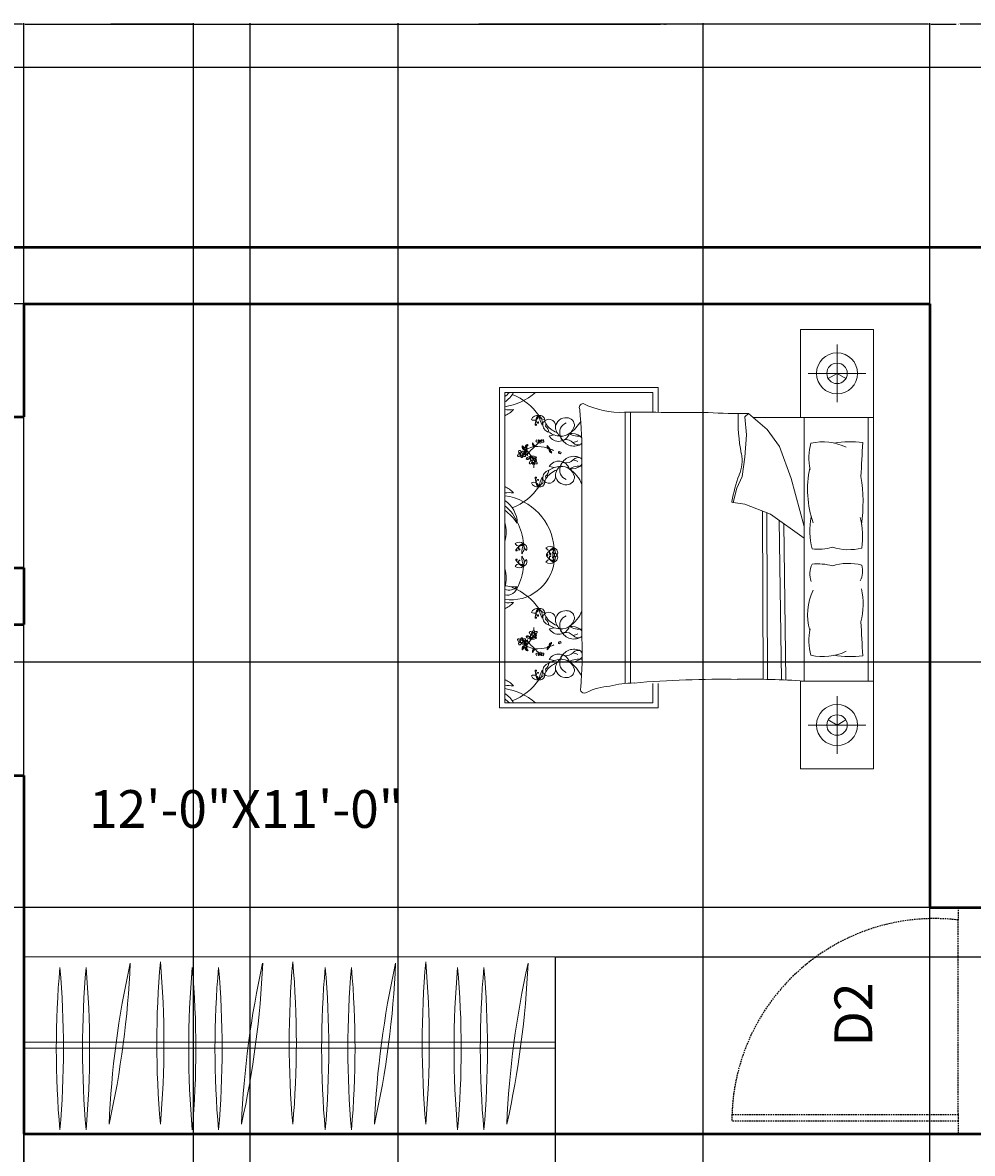
# Model space of a CAD drawing. Units: inches. Extents: x 3 to 576, y -689 to 51.
# Tile 17 of 21: x 111 to 262, y -128 to 51. Entities that reach past the tile are written whole.
import ezdxf

# ---------------------------------------------------------------- set-up
doc = ezdxf.new("R2010")
doc.units = ezdxf.units.IN
doc.header["$MEASUREMENT"] = 0
doc.linetypes.add('DASHED2', pattern=[0.375, 0.25, -0.125])
for name, color, linetype, lineweight in [('A-ANNO-DIMS', 2, 'Continuous', 18), ('A-ANNO-TEXT', 3, 'Continuous', 18), ('A-AREA-IDEN', 7, 'Continuous', 18), ('A-DOOR', 4, 'DASHED2', 25), ('A-FURN', 8, 'Continuous', 18), ('A-WALL', 7, 'Continuous', 50)]:
    doc.layers.add(name, color=color, linetype=linetype, lineweight=lineweight)
doc.styles.get("Standard").update_dxf_attribs({"font": 'arial.ttf'})
doc.dimstyles.get("Standard").update_dxf_attribs({"dimtxt": 0.18, "dimasz": 0.18, "dimexe": 0.18, "dimexo": 0.0625, "dimgap": 0.09, "dimtad": 0, "dimtih": 1, "dimtoh": 1, "dimdec": 0, "dimzin": 0, "dimdsep": 46, "dimlunit": 3, "dimtxsty": 'Standard', "dimcen": 0.09, "dimadec": 0, "dimazin": 0, "dimtfac": 1, "dimtdec": 0, "dimtofl": 0, "dimtmove": 0, "dimatfit": 3, "dimfxl": 1, "dimtolj": 1, "dimtzin": 0, "dimarcsym": 0})

# ---------------------------------------------------------------- blocks, each defined once
blk = doc.blocks.new('*D1')
at = {"layer": 'A-ANNO-DIMS', "color": 0, "lineweight": -2, "transparency": 16777216}
for p, q in [((38.29, 15.75), (38.29, 44.49)), ((38.47, 44.31), (276.45, 44.31)), ((540.11, 44.31), (302.14, 44.31)), ((540.29, 15.75), (540.29, 44.49))]:
    blk.add_line(p, q, dxfattribs=at)
at = {"layer": 'A-ANNO-DIMS', "color": 0, "transparency": 16777216}
for points in [[(38.47, 44.34), (38.47, 44.28), (38.29, 44.31)], [(540.11, 44.34), (540.11, 44.28), (540.29, 44.31)]]:
    blk.add_solid(points, dxfattribs=at)
at = {"layer": 'Defpoints', "color": 0, "transparency": 16777216}
for p in [(540.29, 44.31), (38.29, 15.69), (540.29, 15.69)]:
    blk.add_point(p, dxfattribs=at)
at = {"layer": 'A-ANNO-DIMS', "color": 0, "transparency": 16777216, "insert": (289.29, 44.31), "char_height": 6, "attachment_point": 5}
blk.add_mtext('\\A1;41\'-10"', dxfattribs=at)
blk = doc.blocks.new('BED-DOUBLE')
for p, q in [((59.45, 69.91), (59.45, 0)), ((53.63, 58.35), (53.63, 67.49)), ((49.06, 62.92), (58.2, 62.92)), ((0, 60.68), (25.18, 60.68)), ((0, 9.72), (0, 60.68)), ((0.81, 59.87), (0.81, 10.53)), ((24.37, 59.87), (0.81, 59.87)), ((24.37, 56.73), (24.37, 59.87)), ((25.18, 60.68), (25.18, 56.73)), ((19.95, 13.6), (19.95, 56.73)), ((20.82, 13.66), (20.82, 56.73)), ((38.97, 55.99), (39.54, 56.55)), ((39.25, 53.16), (38.97, 55.99)), ((39.54, 56.55), (42.51, 54.01)), ((59.45, 55.93), (40.27, 55.93)), ((48.41, 55.93), (48.41, 13.98)), ((58.56, 13.98), (58.56, 55.93)), ((42.51, 54.01), (44.49, 51.31)), ((7.9, 52.98), (8.69, 53.14)), ((38.97, 49.62), (39.25, 53.16)), ((44.49, 51.31), (46.33, 46.22)), ((13.08, 20.76), (13.08, 49.15)), ((38.55, 46.5), (38.97, 49.62)), ((7.9, 48.1), (8.69, 47.94)), ((37.7, 44.66), (38.55, 46.5)), ((46.33, 46.22), (48.41, 38.59)), ((37.13, 42.39), (37.7, 44.66)), ((38.97, 42.11), (37.13, 42.39)), ((43.07, 40.55), (38.97, 42.11)), ((41.87, 14.23), (41.76, 41.05)), ((42.58, 14.23), (42.48, 40.78)), ((48.41, 36.72), (43.07, 40.55)), ((44.78, 14.2), (44.43, 39.58)), ((45.5, 14.17), (45.15, 39.06)), ((7.9, 22.3), (8.69, 22.46)), ((7.9, 17.41), (8.69, 17.26)), ((24.37, 10.53), (24.37, 13.61)), ((25.18, 13.59), (25.18, 9.72)), ((53.63, 11.56), (53.63, 2.42)), ((25.18, 9.72), (0, 9.72)), ((0.81, 10.53), (24.37, 10.53)), ((49.06, 6.99), (58.2, 6.99))]:
    blk.add_line(p, q)
for points in [[(47.8, 55.93), (47.8, 69.91), (59.45, 69.91)], [(53.63, 62.92), (52.22, 62.1)], [(53.63, 62.92), (55.04, 62.1)], [(59.45, 13.98), (47.8, 13.98), (47.8, 0), (59.45, 0)], [(53.63, 6.99), (52.22, 7.81)], [(53.63, 6.99), (55.04, 7.81)]]:
    blk.add_lwpolyline(points)
for points in [[(33.13, 56.7, 0.001242), (19.87, 56.73, -0.127202), (13.26, 58.14)], [(57.71, 51.91, 0.074897), (53.14, 51.83, -0.472817)], [(52.89, 35.28, 0.14099), (57.55, 35.14, 0.235245)], [(52.89, 32.3, -0.14099), (57.55, 32.44, -0.235245)], [(57.71, 18, -0.074897), (53.14, 18.08, 0.472817)], [(21.37, 13.68, 0.056112), (17.53, 13.18, 0.095341), (13.82, 12.19)]]:
    blk.add_lwpolyline(points, format="xyb")
for centre, radius in [((53.63, 62.92), 3.26), ((53.63, 62.92), 1.63), ((3.49, 50.11), 0.178), ((5.36, 48.94), 0.178), ((5.36, 21.45), 0.178), ((3.49, 20.29), 0.178), ((53.63, 6.99), 3.26), ((53.63, 6.99), 1.63)]:
    blk.add_circle(centre, radius)
for centre, radius, start, end in [((-2.47, 63.69), 5.54, 306.3036, 316.4814), ((-1.64, 62.09), 4.45, 303.4617, 330.1116), ((-0.42, 66.67), 9.13, 277.745, 311.8856), ((-1.32, 51.05), 9.13, 34.3865, 68.5908), ((13.3, 57.49), 0.645, 93.98, 207.3412), ((-0.61, 59.6), 3.71, 292.5547, 318.9546), ((1.38, 69.77), 12.63, 267.4081, 273.6519), ((6, 55.22), 1.01, 77.7115, 159.0387), ((5.45, 56.23), 0.762, 238.4633, 358.2869), ((7.95, 54.69), 2.31, 138.8402, 177.9352), ((6.56, 55.55), 0.747, 117.6827, 223.7762), ((6.39, 55.47), 0.757, 2.9516, 103.728), ((12.45, 57.59), 6.39, 192.5173, 207.1824), ((5.37, 55.04), 1.44, 345.4653, 54.2343), ((7.54, 57.02), 1.56, 211.3827, 255.2969), ((10.53, 54.2), 1.67, 84.9449, 172.8857), ((10.7, 54.68), 1.18, 354.4856, 91.0538), ((-59.69, 49.98), 72.78, 359.3433, 5.6887), ((37.8, 120.65), 64.12, 265.8294, 271.553), ((64.29, 55.36), 26.39, 177.4519, 191.3392), ((5.76, 54.77), 0.113, 177.9352, 11.4834), ((5.81, 54.78), 0.0551, 11.4834, 127.9409), ((6.09, 55.1), 0.0988, 223.7762, 159.7183), ((7.84, 54.58), 1.05, 350.264, 160.8688), ((8.16, 54.83), 1.31, 175.969, 254.3045), ((6.7, 54.8), 0.643, 333.9755, 53.2681), ((6.41, 53.42), 1.4, 6.1662, 51.5825), ((10.15, 56.66), 3.3, 211.2614, 251.7045), ((10.9, 54.49), 2.03, 182.3591, 234.0401), ((11.17, 53.54), 1.62, 111.5819, 201.4221), ((9.83, 55.04), 2.1, 265.2933, 346.921), ((8.16, 57.76), 5.29, 303.6671, 333.2997), ((5.91, 52.13), 0.137, 142.4737, 265.053), ((6.09, 52.15), 0.294, 127.7621, 169.0403), ((5.94, 52.4), 0.414, 265.053, 338.3618), ((6.48, 51.84), 0.541, 113.4276, 137.6104), ((6.42, 52.4), 0.178, 183.2768, 356.7232), ((6.55, 52.07), 0.291, 139.7889, 227.6792), ((5.87, 52.08), 0.583, 353.0852, 15.7171), ((6.25, 52.01), 0.368, 350.3487, 43.6538), ((6.93, 52.39), 0.428, 198.7263, 262.5032), ((6.59, 52.19), 0.17, 1.1081, 91.8675), ((6.91, 52.1), 0.138, 255.2356, 54.9248), ((6.7, 52.15), 0.297, 11.5637, 52.6358), ((9.88, 56.69), 3.75, 236.2883, 266.5076), ((9.4, 53.85), 1.74, 209.9085, 343.1337), ((10.13, 52.75), 0.434, 167.3041, 285.1471), ((11.31, 50.67), 2.7, 122.7011, 126.3445), ((11.81, 53.58), 2.23, 199.2822, 299.1751), ((10.62, 50.95), 1.43, 41.5653, 105.1471), ((12.57, 55.82), 2.9, 238.8218, 279.1554), ((11.31, 50.67), 2.7, 55.785, 94.7304), ((11.41, 53.92), 2.01, 277.436, 299.9149), ((12.31, 52.24), 0.842, 30.0293, 52.325), ((3.35, 50.47), 0.351, 157.4086, 261.4386), ((3.15, 50.48), 0.176, 58.0499, 135.6268), ((3.34, 50.37), 0.118, 172.906, 277.132), ((2.95, 50.16), 0.561, 14.7558, 58.0499), ((3.74, 50.31), 0.243, 36.1046, 181.4281), ((3.75, 51.26), 0.199, 124.3538, 214.3923), ((4.04, 51.23), 0.464, 190.3057, 287.1958), ((3.59, 50.5), 0.245, 270.0645, 331.1507), ((4.17, 51.39), 0.538, 176.9701, 248.2913), ((8.01, 54.23), 5.2, 212.6784, 216.3746), ((3.8, 50.33), 0.174, 263.7526, 41.7054), ((3.99, 51.27), 0.206, 216.3746, 291.7548), ((5.81, 48.38), 2.9, 124.0033, 132.4917), ((2.83, 48.01), 3.1, 63.7819, 68.2913), ((4.48, 50.4), 0.493, 128.3208, 208.8162), ((4.48, 51.12), 0.464, 122.8155, 187.3992), ((4.12, 50.93), 0.155, 289.3605, 111.7548), ((4.24, 50.93), 0.155, 221.8703, 44.2646), ((4.94, 50.48), 0.812, 157.2305, 229.0635), ((4.69, 51.06), 0.538, 109.4799, 177.6828), ((4.67, 50.75), 0.478, 174.4544, 220.6188), ((1.96, 48.08), 3.48, 30.544, 49.818), ((4.4, 51.4), 0.199, 56.8636, 146.9021), ((4.5, 51.18), 0.206, 148.8844, 224.2646), ((3.87, 50.06), 0.574, 340.0041, 40.6188), ((8.78, 48.6), 5.2, 145.1882, 148.8844), ((5.81, 48.38), 2.9, 94.756, 119.2041), ((11.99, 44.2), 9.55, 132.2412, 142.1744), ((7.17, 51.8), 1.97, 178.3264, 187.1302), ((5.04, 51.53), 0.367, 11.3256, 64.4621), ((6.29, 52.06), 1.1, 190.2588, 210.656), ((5.55, 51.61), 0.336, 188.3432, 274.2869), ((5.84, 51.79), 0.586, 210.656, 242.6341), ((6.28, 52.3), 1.12, 218.2101, 226.3071), ((5.45, 51.35), 0.142, 325.7657, 67.4417), ((1.03, 56.11), 6.64, 313.1541, 322.0459), ((5.96, 45.49), 5.79, 73.5842, 93.8277), ((6.46, 51.97), 0.153, 227.6792, 350.3487), ((9.52, 51.39), 1.97, 178.3264, 187.1302), ((7.39, 51.11), 0.367, 11.3256, 64.4621), ((8.64, 51.64), 1.1, 190.2588, 210.656), ((7.9, 51.19), 0.336, 188.3432, 274.2869), ((8.19, 51.38), 0.586, 210.656, 242.6341), ((8.64, 51.88), 1.12, 218.2101, 226.3071), ((7.81, 50.93), 0.142, 325.7657, 67.4417), ((8.21, 50.67), 0.336, 147.5332, 233.4768), ((7.94, 50.71), 0.142, 354.3784, 96.0543), ((8.51, 50.85), 0.586, 179.1859, 211.164), ((5.96, 45.49), 5.79, 63.0032, 69.8941), ((8.95, 51.12), 1.1, 211.164, 231.5612), ((9.15, 52.01), 1.97, 234.6898, 243.4936), ((9.16, 51), 1.12, 195.5129, 203.6099), ((7.9, 50.27), 0.367, 357.3579, 50.4944), ((9.48, 50.34), 0.135, 12.7051, 190.4384), ((9.56, 50.36), 0.219, 190.4384, 10.4136), ((12.48, 52.59), 1.05, 221.5653, 293.8354), ((12.31, 52.24), 0.842, 314.4517, 333.558), ((58.53, 49.42), 9.37, 165.1039, 191.0369), ((51.31, 43.01), 9.01, 65.1316, 101.7583), ((723.03, 13.38), 666.43, 176.68521, 177.14978), ((2.98, 49.84), 0.137, 142.4737, 265.053), ((3.16, 49.87), 0.294, 61.2196, 169.0403), ((3, 50.12), 0.414, 265.053, 338.3618), ((3.55, 49.55), 0.541, 113.4276, 137.6104), ((3.62, 49.79), 0.291, 139.7889, 227.6792), ((3.53, 49.68), 0.153, 227.6792, 350.3487), ((2.93, 49.79), 0.583, 353.0852, 15.7171), ((3.31, 49.72), 0.368, 350.3487, 43.6538), ((3.8, 50.44), 0.28, 221.8413, 265.7877), ((4, 50.1), 0.428, 198.7263, 262.5032), ((3.66, 49.9), 0.17, 1.1081, 91.8675), ((3.76, 49.86), 0.297, 11.5637, 86.365), ((3.98, 49.81), 0.138, 255.2356, 54.9248), ((4.57, 50.43), 0.59, 207.7043, 254.3516), ((4.19, 50.1), 0.812, 270.278, 342.111), ((4.73, 49.08), 0.574, 98.7227, 159.3375), ((4.44, 49.82), 0.59, 244.9899, 291.6373), ((4.57, 50.12), 0.478, 278.7227, 324.8872), ((4.49, 49.73), 0.493, 290.5253, 358.5375), ((4.85, 48.67), 0.137, 142.4737, 265.053), ((5.03, 48.7), 0.294, 61.2196, 169.0403), ((4.88, 48.95), 0.414, 265.053, 338.3618), ((5.23, 49.31), 0.351, 157.4086, 261.4386), ((5.03, 49.32), 0.176, 58.0499, 135.6268), ((5.45, 49.87), 0.493, 182.8499, 266.1226), ((5.26, 50.22), 0.478, 231.7607, 277.9252), ((5.63, 50.31), 0.812, 214.5369, 286.3699), ((5.43, 48.38), 0.541, 113.4276, 137.6104), ((5.21, 49.21), 0.118, 172.906, 277.132), ((4.83, 48.99), 0.561, 14.7558, 58.0499), ((1.96, 48.08), 3.48, 23.0501, 23.8477), ((5.5, 48.62), 0.291, 139.7889, 227.6792), ((5.4, 49.18), 0.574, 37.3105, 97.9252), ((5.61, 49.14), 0.243, 36.1046, 181.4281), ((4.81, 48.63), 0.583, 353.0852, 15.7171), ((5.47, 49.97), 0.59, 265.0106, 311.658), ((5.19, 48.56), 0.368, 350.3487, 43.6538), ((5.47, 49.33), 0.245, 270.0645, 331.1507), ((5.68, 49.27), 0.28, 221.8413, 265.7877), ((5.87, 48.94), 0.428, 198.7263, 262.5032), ((5.53, 48.74), 0.17, 1.1081, 91.8675), ((5.68, 49.17), 0.174, 263.7526, 41.7054), ((5.64, 48.7), 0.297, 11.5637, 86.365), ((5.85, 48.65), 0.138, 255.2356, 54.9248), ((9.4, 47.23), 1.74, 16.8663, 150.0915), ((10.13, 48.33), 0.434, 74.8529, 192.6959), ((11.81, 47.5), 2.23, 60.8249, 160.7178), ((10.62, 50.13), 1.43, 254.8529, 318.4347), ((11.41, 47.16), 2.01, 60.0851, 82.564), ((12.48, 48.49), 1.05, 66.1646, 138.4347), ((12.31, 48.84), 0.842, 23.229, 45.5483), ((32.84, 49.05), 5.69, 336.2616, 11.3392), ((5.4, 48.52), 0.153, 227.6792, 350.3487), ((1.96, 48.08), 3.48, 357.1071, 4.7585), ((8.16, 46.25), 1.31, 105.6955, 184.031), ((6.41, 47.66), 1.4, 308.4175, 353.8338), ((10.15, 44.42), 3.3, 108.2955, 148.7386), ((9.88, 44.39), 3.75, 93.4924, 123.7117), ((10.9, 46.59), 2.03, 125.9599, 177.6409), ((11.17, 47.54), 1.62, 158.5779, 248.4181), ((9.83, 46.04), 2.1, 13.079, 94.7067), ((11.31, 50.41), 2.7, 233.6555, 237.2989), ((12.57, 45.26), 2.9, 79.7133, 121.1782), ((11.31, 50.41), 2.7, 265.2696, 304.215), ((8.16, 43.32), 5.29, 21.4941, 56.3329), ((12.31, 48.84), 0.842, 307.675, 336.7144), ((63.55, 37.54), 27.11, 160.1194, 169.3383), ((65.19, 44.49), 16.25, 168.0397, 199.2615), ((5.45, 44.85), 0.762, 1.7131, 121.5367), ((6, 45.86), 1.01, 200.9613, 282.2885), ((5.76, 46.31), 0.113, 348.5166, 182.0648), ((7.95, 46.39), 2.31, 182.0648, 221.1598), ((5.81, 46.3), 0.0551, 232.0591, 348.5166), ((6.56, 45.54), 0.747, 136.2238, 242.3173), ((6.13, 45.97), 0.0595, 200.2667, 136.2271), ((5.37, 46.05), 1.44, 305.7657, 14.5347), ((12.45, 43.49), 6.39, 152.8176, 167.4827), ((6.39, 45.61), 0.757, 256.272, 357.0484), ((7.54, 44.06), 1.56, 104.7031, 148.6173), ((7.84, 46.5), 1.05, 199.1312, 9.736), ((6.7, 46.28), 0.643, 306.7319, 26.0245), ((10.53, 46.88), 1.67, 187.1143, 275.0551), ((10.7, 46.4), 1.18, 268.9462, 5.5144), ((32.41, 42.33), 25.35, 352.2196, 9.497), ((-0.61, 41.48), 3.71, 41.0454, 67.4453), ((1.38, 31.32), 12.63, 86.3481, 92.5919), ((-0.42, 34.41), 9.13, 4.4623, 82.255), ((-1.32, 50.03), 9.13, 291.4092, 325.6135), ((-1.64, 38.99), 4.45, 1.272, 56.5383), ((-2.47, 37.39), 5.54, 17.8504, 53.6964), ((37.07, 42.55), 0.169, 178.8623, 289.7536), ((-4.03, 34.48), 8.25, 34.0123, 54.053), ((61.64, 37.91), 12.33, 169.8617, 193.6238), ((45.23, 36.98), 12.46, 351.5249, 13.96), ((-3.99, 37.66), 5.02, 343.5431, 17.0202), ((-5.31, 35.11), 9.13, 4.4623, 27.4146), ((-6.58, 35.67), 7.42, 4.3787, 5.6357), ((-11.66, 31.77), 13.27, 19.7217, 19.9028), ((3.11, 35.07), 1.01, 47.7873, 129.1145), ((3.14, 36.22), 0.762, 208.5391, 328.3627), ((2.68, 34.8), 0.113, 148.011, 341.5592), ((4.54, 33.64), 2.31, 108.9159, 148.011), ((2.73, 34.78), 0.0551, 341.5592, 98.0167), ((3.76, 35.07), 0.747, 87.7585, 193.852), ((3.13, 34.92), 0.0988, 193.852, 129.9245), ((9.89, 33.91), 6.39, 162.593, 177.2582), ((2.48, 35.23), 1.44, 315.5411, 24.3101), ((5.35, 35.86), 1.56, 181.4585, 225.3727), ((3.58, 35.09), 0.757, 333.0274, 73.8037), ((8, 34.37), 1.01, 47.7873, 129.1145), ((8.03, 35.52), 0.762, 208.5391, 328.3627), ((9.43, 32.94), 2.31, 108.9159, 148.011), ((8.65, 34.38), 0.747, 87.7585, 193.852), ((8.02, 34.22), 0.0988, 193.852, 129.9245), ((7.37, 34.53), 1.44, 315.5411, 24.3101), ((14.78, 33.21), 6.39, 162.593, 177.2582), ((7.37, 33.54), 1.44, 335.6899, 44.4589), ((14.78, 34.86), 6.39, 182.7418, 197.407), ((8.47, 34.4), 0.757, 333.0274, 73.8037), ((10.24, 35.16), 1.56, 181.4585, 225.3727), ((50.55, 43.52), 8.57, 264.0129, 285.8293), ((1.69, 33.95), 7.07, 262.8636, 351.8197), ((3.14, 31.85), 0.762, 31.6373, 151.4609), ((2.68, 33.27), 0.113, 18.4408, 211.989), ((4.54, 34.43), 2.31, 211.989, 251.0841), ((2.73, 33.29), 0.0551, 261.9833, 18.4408), ((3.76, 32.99), 0.747, 166.148, 272.2415), ((3.17, 33.16), 0.0595, 230.1909, 166.0209), ((9.89, 34.16), 6.39, 182.7418, 197.407), ((2.48, 32.84), 1.44, 335.6899, 44.4589), ((5.35, 32.21), 1.56, 134.6273, 178.5415), ((3.58, 32.97), 0.757, 286.1963, 26.9726), ((8.03, 32.55), 0.762, 31.6373, 151.4609), ((8, 33.7), 1.01, 230.8855, 312.2127), ((7.57, 34.1), 0.113, 148.011, 341.5592), ((7.57, 33.97), 0.113, 18.4408, 211.989), ((9.43, 35.13), 2.31, 211.989, 251.0841), ((7.62, 34.08), 0.0551, 341.5592, 98.0167), ((7.62, 33.99), 0.0551, 261.9833, 18.4408), ((8.65, 33.69), 0.747, 166.148, 272.2415), ((8.06, 33.86), 0.0595, 230.1909, 166.0209), ((8.47, 33.67), 0.757, 286.1963, 26.9726), ((10.24, 32.91), 1.56, 134.6273, 178.5415), ((53.02, 31.01), 3.71, 155.0183, 198.5407), ((50.55, 24.06), 8.57, 74.1707, 95.9871), ((54.23, 31.48), 3.46, 333.3437, 16.1026), ((-3.99, 30.4), 5.02, 342.9798, 16.4569), ((-6.58, 32.39), 7.42, 354.3643, 355.6213), ((-11.66, 36.3), 13.27, 340.0972, 340.2783), ((3.11, 33), 1.01, 230.8855, 312.2127), ((-5.31, 32.96), 9.13, 332.5854, 355.5377), ((2.33, 33.04), 4.09, 248.117, 276.6195), ((1.2, 29.29), 1.64, 256.3898, 349.0739), ((1.42, 30.52), 2.07, 252.8609, 311.9049), ((-1.32, 20.37), 9.13, 34.3865, 68.5908), ((57.84, 24.53), 8.9, 153.8761, 196.1746), ((45.48, 26.29), 12.29, 346.3427, 11.1841), ((1.38, 39.08), 12.63, 267.4081, 273.6519), ((-0.61, 28.92), 3.71, 292.5547, 318.9546), ((6, 24.53), 1.01, 77.7115, 159.0387), ((5.45, 25.55), 0.762, 238.4633, 358.2869), ((7.95, 24), 2.31, 138.8402, 177.9352), ((6.56, 24.86), 0.747, 117.6827, 223.7762), ((6.39, 24.79), 0.757, 2.9516, 103.728), ((7.54, 26.34), 1.56, 211.3827, 255.2969), ((5.37, 24.35), 1.44, 345.4653, 54.2343), ((12.45, 26.91), 6.39, 192.5173, 207.1824), ((10.53, 23.52), 1.67, 84.9449, 172.8857), ((10.7, 24), 1.18, 354.4856, 91.0538), ((5.76, 24.08), 0.113, 177.9352, 11.4834), ((5.81, 24.09), 0.0551, 11.4834, 127.9409), ((6.09, 24.41), 0.0988, 223.7762, 159.7183), ((7.84, 23.9), 1.05, 350.264, 160.8688), ((8.16, 24.15), 1.31, 175.969, 254.3045), ((6.7, 24.12), 0.643, 333.9755, 53.2681), ((6.41, 22.74), 1.4, 6.1662, 51.5825), ((10.15, 25.98), 3.3, 211.2614, 251.7045), ((10.9, 23.81), 2.03, 182.3591, 234.0401), ((11.17, 22.86), 1.62, 111.5819, 201.4221), ((9.83, 24.36), 2.1, 265.2933, 346.921), ((8.16, 27.08), 5.29, 303.6671, 338.5059), ((723.03, 56.53), 666.43, 182.85022, 183.31479), ((4.85, 21.72), 0.137, 94.947, 217.5263), ((5.03, 21.7), 0.294, 190.9597, 298.7804), ((4.88, 21.45), 0.414, 21.6382, 94.947), ((5.43, 22.01), 0.541, 222.3896, 246.5724), ((5.5, 21.78), 0.291, 132.3208, 220.2111), ((5.4, 21.88), 0.153, 9.6513, 132.3208), ((4.81, 21.77), 0.583, 344.2829, 6.9148), ((1.96, 22.32), 3.48, 355.2415, 2.8929), ((5.19, 21.84), 0.368, 316.3462, 9.6513), ((5.87, 21.46), 0.428, 97.4968, 161.2737), ((5.53, 21.66), 0.17, 268.1325, 358.8919), ((5.64, 21.7), 0.297, 273.635, 348.4363), ((5.85, 21.75), 0.138, 305.0752, 104.7644), ((9.88, 26.01), 3.75, 236.2883, 266.5076), ((9.4, 23.17), 1.74, 209.9085, 343.1337), ((10.13, 22.07), 0.434, 167.3041, 285.1471), ((11.31, 19.99), 2.7, 122.7011, 126.3445), ((11.81, 22.9), 2.23, 199.2822, 299.1751), ((10.62, 20.26), 1.43, 41.5653, 105.1471), ((12.57, 25.14), 2.9, 238.8218, 280.2867), ((11.31, 19.99), 2.7, 55.785, 94.7304), ((12.31, 21.55), 0.842, 23.2856, 52.325), ((58.53, 20.49), 9.37, 168.9631, 194.8961), ((2.98, 20.56), 0.137, 94.947, 217.5263), ((3.16, 20.53), 0.294, 190.9597, 298.7804), ((3, 20.28), 0.414, 21.6382, 94.947), ((3.35, 19.93), 0.351, 98.5614, 202.5914), ((3.15, 19.91), 0.176, 224.3732, 301.9501), ((3.55, 20.85), 0.541, 222.3896, 246.5724), ((3.34, 20.03), 0.118, 82.868, 187.094), ((2.95, 20.24), 0.561, 301.9501, 345.2442), ((3.62, 20.61), 0.291, 132.3208, 220.2111), ((3.53, 20.71), 0.153, 9.6513, 132.3208), ((2.93, 20.61), 0.583, 344.2829, 6.9148), ((3.74, 20.09), 0.243, 178.5719, 323.8954), ((3.31, 20.68), 0.368, 316.3462, 9.6513), ((4, 20.3), 0.428, 97.4968, 161.2737), ((3.8, 19.96), 0.28, 94.2123, 138.1587), ((3.59, 19.9), 0.245, 28.8493, 89.9355), ((3.66, 20.5), 0.17, 268.1325, 358.8919), ((3.76, 20.54), 0.297, 273.635, 348.4363), ((3.8, 20.07), 0.174, 318.2946, 96.2474), ((5.81, 22.02), 2.9, 227.5083, 235.9967), ((3.98, 20.59), 0.138, 305.0752, 104.7644), ((4.48, 20), 0.493, 151.1838, 231.6792), ((4.57, 19.96), 0.59, 105.6484, 152.2957), ((4.94, 19.92), 0.812, 130.9365, 202.7695), ((4.44, 20.58), 0.59, 68.3627, 115.0101), ((4.19, 20.3), 0.812, 17.889, 89.722), ((4.73, 21.32), 0.574, 200.6625, 261.2773), ((4.67, 19.65), 0.478, 139.3812, 185.5456), ((1.96, 22.32), 3.48, 310.182, 329.456), ((3.87, 20.33), 0.574, 319.3812, 19.9959), ((11.99, 26.2), 9.55, 217.8256, 227.7588), ((4.57, 20.28), 0.478, 35.1128, 81.2773), ((4.49, 20.66), 0.493, 1.4625, 69.4747), ((5.23, 21.09), 0.351, 98.5614, 202.5914), ((5.03, 21.08), 0.176, 224.3732, 301.9501), ((5.45, 20.52), 0.493, 93.8774, 177.1501), ((5.63, 20.09), 0.812, 73.6301, 145.4631), ((5.26, 20.18), 0.478, 82.0748, 128.2393), ((5.21, 21.19), 0.118, 82.868, 187.094), ((4.83, 21.41), 0.561, 301.9501, 345.2442), ((1.96, 22.32), 3.48, 336.1523, 336.9499), ((5.4, 21.22), 0.574, 262.0748, 322.6895), ((5.61, 21.26), 0.243, 178.5719, 323.8954), ((5.47, 20.43), 0.59, 48.342, 94.9894), ((5.68, 21.12), 0.28, 94.2123, 138.1587), ((5.47, 21.07), 0.245, 28.8493, 89.9355), ((5.68, 21.23), 0.174, 318.2946, 96.2474), ((8.21, 19.72), 0.336, 126.5232, 212.4668), ((8.51, 19.55), 0.586, 148.836, 180.8141), ((8.95, 19.28), 1.1, 128.4388, 148.836), ((9.15, 18.38), 1.97, 116.5064, 125.3102), ((9.16, 19.4), 1.12, 156.3901, 164.4871), ((7.9, 20.13), 0.367, 309.5056, 2.6421), ((9.56, 20.04), 0.219, 349.5864, 169.5616), ((9.48, 20.06), 0.135, 169.5616, 347.2949), ((11.41, 23.23), 2.01, 277.436, 299.9149), ((12.48, 21.91), 1.05, 221.5653, 293.8354), ((-54.91, 18.62), 68.03, 355.2402, 1.8035), ((12.31, 21.55), 0.842, 314.4517, 336.7144), ((3.75, 19.14), 0.199, 145.6077, 235.6462), ((4.04, 19.17), 0.464, 72.8042, 169.6943), ((4.17, 19.01), 0.538, 111.7087, 183.0299), ((8.01, 16.17), 5.2, 143.6254, 147.3216), ((3.99, 19.13), 0.206, 68.2452, 143.6254), ((2.83, 22.39), 3.1, 291.7087, 296.2181), ((4.48, 19.27), 0.464, 172.6008, 237.1845), ((4.12, 19.47), 0.155, 248.2452, 70.6395), ((4.24, 19.47), 0.155, 315.7354, 138.1297), ((4.69, 19.33), 0.538, 182.3172, 250.5201), ((4.4, 18.99), 0.199, 213.0979, 303.1364), ((4.5, 19.21), 0.206, 135.7354, 211.1156), ((8.78, 21.8), 5.2, 211.1156, 214.8118), ((5.81, 22.02), 2.9, 240.7959, 265.244), ((6.29, 18.34), 1.1, 149.344, 169.7412), ((7.17, 18.6), 1.97, 172.8698, 181.6736), ((5.04, 18.87), 0.367, 295.5379, 348.6744), ((5.55, 18.79), 0.336, 85.7131, 171.6568), ((5.84, 18.61), 0.586, 117.3659, 149.344), ((6.28, 18.1), 1.12, 133.6929, 141.7899), ((5.45, 19.05), 0.142, 292.5583, 34.2343), ((5.96, 24.9), 5.79, 266.1723, 286.4158), ((1.03, 14.28), 6.64, 37.9541, 46.8459), ((5.91, 18.27), 0.137, 94.947, 217.5263), ((6.09, 18.24), 0.294, 190.9597, 232.2379), ((5.94, 18), 0.414, 21.6382, 94.947), ((6.48, 18.56), 0.541, 222.3896, 246.5724), ((6.42, 18), 0.178, 3.2768, 176.7232), ((6.55, 18.32), 0.291, 132.3208, 220.2111), ((6.46, 18.43), 0.153, 9.6513, 132.3208), ((5.87, 18.32), 0.583, 344.2829, 6.9148), ((6.25, 18.39), 0.368, 316.3462, 9.6513), ((6.93, 18.01), 0.428, 97.4968, 161.2737), ((6.59, 18.21), 0.17, 268.1325, 358.8919), ((6.91, 18.3), 0.138, 305.0752, 104.7644), ((6.7, 18.25), 0.297, 307.3642, 348.4363), ((8.64, 18.76), 1.1, 149.344, 169.7412), ((9.52, 19.01), 1.97, 172.8698, 181.6736), ((7.39, 19.29), 0.367, 295.5379, 348.6744), ((7.9, 19.21), 0.336, 85.7131, 171.6568), ((8.19, 19.02), 0.586, 117.3659, 149.344), ((8.64, 18.52), 1.12, 133.6929, 141.7899), ((7.81, 19.46), 0.142, 292.5583, 34.2343), ((9.4, 16.55), 1.74, 16.8663, 150.0915), ((7.94, 19.68), 0.142, 263.9457, 5.6216), ((5.96, 24.9), 5.79, 290.1059, 296.9968), ((10.13, 17.65), 0.434, 74.8529, 192.6959), ((11.81, 16.82), 2.23, 60.8249, 160.7178), ((10.62, 19.45), 1.43, 254.8529, 318.4347), ((11.41, 16.48), 2.01, 60.0851, 82.564), ((12.48, 17.81), 1.05, 66.1646, 138.4347), ((12.31, 18.16), 0.842, 16.6343, 45.5483), ((51.31, 26.9), 9.01, 258.2417, 294.8684), ((8.16, 15.56), 1.31, 105.6955, 184.031), ((6.41, 16.98), 1.4, 308.4175, 353.8338), ((10.15, 13.74), 3.3, 108.2955, 148.7386), ((9.88, 13.7), 3.75, 93.4924, 123.7117), ((10.9, 15.91), 2.03, 125.9599, 177.6409), ((11.17, 16.86), 1.62, 158.5779, 248.4181), ((9.83, 15.35), 2.1, 13.079, 94.7067), ((11.31, 19.72), 2.7, 233.6555, 237.2989), ((12.57, 14.57), 2.9, 79.249, 121.1782), ((11.31, 19.72), 2.7, 265.2696, 304.215), ((8.16, 12.63), 5.29, 23.6453, 56.3329), ((12.31, 18.16), 0.842, 307.675, 342.5814), ((5.45, 14.17), 0.762, 1.7131, 121.5367), ((6, 15.18), 1.01, 200.9613, 282.2885), ((5.76, 15.63), 0.113, 348.5166, 182.0648), ((7.95, 15.71), 2.31, 182.0648, 221.1598), ((5.81, 15.62), 0.0551, 232.0591, 348.5166), ((6.56, 14.85), 0.747, 136.2238, 242.3173), ((6.13, 15.29), 0.0595, 200.2667, 136.2271), ((12.45, 12.81), 6.39, 152.8176, 167.4827), ((5.37, 15.36), 1.44, 305.7657, 14.5347), ((7.54, 13.38), 1.56, 104.7031, 148.6173), ((6.39, 14.93), 0.757, 256.272, 357.0484), ((7.84, 15.82), 1.05, 199.1312, 9.736), ((6.7, 15.6), 0.643, 306.7319, 26.0245), ((10.53, 16.2), 1.67, 187.1143, 275.0551), ((10.7, 15.72), 1.18, 268.9462, 5.5144), ((-0.61, 10.8), 3.71, 41.0454, 67.4453), ((1.38, 0.63), 12.63, 86.3481, 92.5919), ((-0.42, 3.73), 9.13, 48.1144, 82.255), ((-1.32, 19.35), 9.13, 291.4092, 325.6135), ((13.47, 12.72), 0.637, 156.5219, 303.8264), ((35.29, -149.59), 163.86, 89.1145, 94.8735), ((39.86, -111.34), 125.62, 86.1, 90.9282), ((-1.64, 8.31), 4.45, 29.8884, 56.5383), ((-2.47, 6.71), 5.54, 43.5186, 53.6964)]:
    blk.add_arc(centre, radius, start, end)
blk = doc.blocks.new('DOOR-SWING-900')
for p, q in [((35.95, 36), (35.95, 34)), ((36, 2), (35.95, 34)), ((36, 2), (0, 2)), ((36, 0), (36, 2))]:
    blk.add_line(p, q)
blk.add_arc((32.22, 2), 32.22, 83.347, 180)
blk = doc.blocks.new('*D41')
at = {"layer": 'A-ANNO-DIMS', "color": 0, "lineweight": -2, "transparency": 16777216}
for p, q in [((102.29, 15.75), (102.29, 51.32)), ((102.47, 51.14), (106.46, 51.14)), ((111.11, 51.14), (107.12, 51.14)), ((111.29, 6.75), (111.29, 51.32))]:
    blk.add_line(p, q, dxfattribs=at)
at = {"layer": 'A-ANNO-DIMS', "color": 0, "transparency": 16777216}
for points in [[(102.47, 51.17), (102.47, 51.11), (102.29, 51.14)], [(111.11, 51.17), (111.11, 51.11), (111.29, 51.14)]]:
    blk.add_solid(points, dxfattribs=at)
at = {"layer": 'Defpoints', "color": 0, "transparency": 16777216}
for p in [(111.29, 51.14), (102.29, 15.69), (111.29, 6.69)]:
    blk.add_point(p, dxfattribs=at)
at = {"layer": 'A-ANNO-DIMS', "color": 0, "transparency": 16777216, "insert": (106.79, 51.14), "char_height": 0.18, "attachment_point": 5}
blk.add_mtext('\\A1;0\'-9"', dxfattribs=at)
blk = doc.blocks.new('*D42')
at = {"layer": 'A-ANNO-DIMS', "color": 0, "lineweight": -2, "transparency": 16777216}
for p, q in [((111.29, 6.75), (111.29, 51.32)), ((111.47, 51.14), (182.9, 51.14)), ((255.11, 51.14), (183.68, 51.14)), ((255.29, 6.75), (255.29, 51.32))]:
    blk.add_line(p, q, dxfattribs=at)
at = {"layer": 'A-ANNO-DIMS', "color": 0, "transparency": 16777216}
for points in [[(111.47, 51.17), (111.47, 51.11), (111.29, 51.14)], [(255.11, 51.17), (255.11, 51.11), (255.29, 51.14)]]:
    blk.add_solid(points, dxfattribs=at)
at = {"layer": 'Defpoints', "color": 0, "transparency": 16777216}
for p in [(255.29, 51.14), (111.29, 6.69), (255.29, 6.69)]:
    blk.add_point(p, dxfattribs=at)
at = {"layer": 'A-ANNO-DIMS', "color": 0, "transparency": 16777216, "insert": (183.29, 51.14), "char_height": 0.18, "attachment_point": 5}
blk.add_mtext('\\A1;12\'-0"', dxfattribs=at)
blk = doc.blocks.new('*D43')
at = {"layer": 'A-ANNO-DIMS', "color": 0, "lineweight": -2, "transparency": 16777216}
for p, q in [((255.29, 6.75), (255.29, 51.32)), ((255.47, 51.14), (259.46, 51.14)), ((264.11, 51.14), (260.12, 51.14)), ((264.29, 6.75), (264.29, 51.32))]:
    blk.add_line(p, q, dxfattribs=at)
at = {"layer": 'A-ANNO-DIMS', "color": 0, "transparency": 16777216}
for points in [[(255.47, 51.17), (255.47, 51.11), (255.29, 51.14)], [(264.11, 51.17), (264.11, 51.11), (264.29, 51.14)]]:
    blk.add_solid(points, dxfattribs=at)
at = {"layer": 'Defpoints', "color": 0, "transparency": 16777216}
for p in [(264.29, 51.14), (255.29, 6.69), (264.29, 6.69)]:
    blk.add_point(p, dxfattribs=at)
at = {"layer": 'A-ANNO-DIMS', "color": 0, "transparency": 16777216, "insert": (259.79, 51.14), "char_height": 0.18, "attachment_point": 5}
blk.add_mtext('\\A1;0\'-9"', dxfattribs=at)
blk = doc.blocks.new('*D64')
at = {"layer": 'A-ANNO-DIMS', "color": 0, "lineweight": -2, "transparency": 16777216}
for p, q in [((540.23, 15.69), (2.66, 15.69)), ((2.84, 15.51), (2.84, -17.13)), ((2.84, -50.13), (2.84, -17.49)), ((531.23, -50.31), (2.66, -50.31))]:
    blk.add_line(p, q, dxfattribs=at)
at = {"layer": 'A-ANNO-DIMS', "color": 0, "transparency": 16777216}
for points in [[(2.81, 15.51), (2.87, 15.51), (2.84, 15.69)], [(2.81, -50.13), (2.87, -50.13), (2.84, -50.31)]]:
    blk.add_solid(points, dxfattribs=at)
at = {"layer": 'Defpoints', "color": 0, "transparency": 16777216}
for p in [(540.29, 15.69), (2.84, -50.31), (531.29, -50.31)]:
    blk.add_point(p, dxfattribs=at)
at = {"layer": 'A-ANNO-DIMS', "color": 0, "transparency": 16777216, "insert": (2.84, -17.31), "char_height": 0.18, "attachment_point": 5}
blk.add_mtext('\\A1;5\'-6"', dxfattribs=at)
blk = doc.blocks.new('*D65')
at = {"layer": 'A-ANNO-DIMS', "color": 0, "lineweight": -2, "transparency": 16777216}
for p, q in [((531.23, -50.31), (2.66, -50.31)), ((2.84, -50.49), (2.84, -116.13)), ((2.84, -182.13), (2.84, -116.49)), ((531.23, -182.31), (2.66, -182.31))]:
    blk.add_line(p, q, dxfattribs=at)
at = {"layer": 'A-ANNO-DIMS', "color": 0, "transparency": 16777216}
for points in [[(2.81, -50.49), (2.87, -50.49), (2.84, -50.31)], [(2.81, -182.13), (2.87, -182.13), (2.84, -182.31)]]:
    blk.add_solid(points, dxfattribs=at)
at = {"layer": 'Defpoints', "color": 0, "transparency": 16777216}
for p in [(531.29, -50.31), (2.84, -182.31), (531.29, -182.31)]:
    blk.add_point(p, dxfattribs=at)
at = {"layer": 'A-ANNO-DIMS', "color": 0, "transparency": 16777216, "insert": (2.84, -116.31), "char_height": 0.18, "attachment_point": 5}
blk.add_mtext('\\A1;11\'-0"', dxfattribs=at)
blk = doc.blocks.new('*D86')
at = {"layer": 'A-ANNO-DIMS', "color": 0, "lineweight": -2, "transparency": 16777216}
for p, q in [((111.29, -97.21), (111.29, -688.94)), ((195.78, -97.21), (195.78, -688.94)), ((111.47, -688.76), (153, -688.76)), ((195.6, -688.76), (154.08, -688.76))]:
    blk.add_line(p, q, dxfattribs=at)
at = {"layer": 'A-ANNO-DIMS', "color": 0, "transparency": 16777216}
for points in [[(111.47, -688.73), (111.47, -688.79), (111.29, -688.76)], [(195.6, -688.73), (195.6, -688.79), (195.78, -688.76)]]:
    blk.add_solid(points, dxfattribs=at)
at = {"layer": 'Defpoints', "color": 0, "transparency": 16777216}
for p in [(111.29, -97.15), (195.78, -97.15), (195.78, -688.76)]:
    blk.add_point(p, dxfattribs=at)
at = {"layer": 'A-ANNO-DIMS', "color": 0, "transparency": 16777216, "insert": (153.54, -688.76), "char_height": 0.18, "attachment_point": 5}
blk.add_mtext('\\A1;7\'-0 1/2"', dxfattribs=at)
blk = doc.blocks.new('*D87')
at = {"layer": 'A-ANNO-DIMS', "color": 0, "lineweight": -2, "transparency": 16777216}
for p, q in [((195.85, -97.15), (575.92, -97.15)), ((575.74, -97.33), (575.74, -111.05)), ((575.74, -125.13), (575.74, -111.41)), ((195.85, -125.31), (575.92, -125.31))]:
    blk.add_line(p, q, dxfattribs=at)
at = {"layer": 'A-ANNO-DIMS', "color": 0, "transparency": 16777216}
for points in [[(575.71, -97.33), (575.77, -97.33), (575.74, -97.15)], [(575.71, -125.13), (575.77, -125.13), (575.74, -125.31)]]:
    blk.add_solid(points, dxfattribs=at)
at = {"layer": 'Defpoints', "color": 0, "transparency": 16777216}
for p in [(195.78, -97.15), (575.74, -97.15), (195.78, -125.31)]:
    blk.add_point(p, dxfattribs=at)
at = {"layer": 'A-ANNO-DIMS', "color": 0, "transparency": 16777216, "insert": (575.74, -111.23), "char_height": 0.18, "attachment_point": 5}
blk.add_mtext('\\A1;2\'-4"', dxfattribs=at)
blk = doc.blocks.new('*D88')
at = {"layer": 'A-ANNO-DIMS', "color": 0, "lineweight": -2, "transparency": 16777216}
for p, q in [((170.8, -226.08), (170.8, 51.32)), ((170.98, 51.14), (212.51, 51.14)), ((255.11, 51.14), (213.59, 51.14)), ((255.29, -226.08), (255.29, 51.32))]:
    blk.add_line(p, q, dxfattribs=at)
at = {"layer": 'A-ANNO-DIMS', "color": 0, "transparency": 16777216}
for points in [[(170.98, 51.17), (170.98, 51.11), (170.8, 51.14)], [(255.11, 51.17), (255.11, 51.11), (255.29, 51.14)]]:
    blk.add_solid(points, dxfattribs=at)
at = {"layer": 'Defpoints', "color": 0, "transparency": 16777216}
for p in [(255.29, 51.14), (170.8, -226.15), (255.29, -226.15)]:
    blk.add_point(p, dxfattribs=at)
at = {"layer": 'A-ANNO-DIMS', "color": 0, "transparency": 16777216, "insert": (213.05, 51.14), "char_height": 0.18, "attachment_point": 5}
blk.add_mtext('\\A1;7\'-0 1/2"', dxfattribs=at)
blk = doc.blocks.new('*D100')
at = {"layer": 'A-ANNO-DIMS', "color": 0, "lineweight": -2, "transparency": 16777216}
for p, q in [((255.23, 6.69), (2.66, 6.69)), ((2.84, 6.51), (2.84, -41.13)), ((2.84, -89.13), (2.84, -41.49)), ((255.23, -89.31), (2.66, -89.31))]:
    blk.add_line(p, q, dxfattribs=at)
at = {"layer": 'A-ANNO-DIMS', "color": 0, "transparency": 16777216}
for points in [[(2.81, 6.51), (2.87, 6.51), (2.84, 6.69)], [(2.81, -89.13), (2.87, -89.13), (2.84, -89.31)]]:
    blk.add_solid(points, dxfattribs=at)
at = {"layer": 'Defpoints', "color": 0, "transparency": 16777216}
for p in [(255.29, 6.69), (2.84, -89.31), (255.29, -89.31)]:
    blk.add_point(p, dxfattribs=at)
at = {"layer": 'A-ANNO-DIMS', "color": 0, "transparency": 16777216, "insert": (2.84, -41.31), "char_height": 0.18, "attachment_point": 5}
blk.add_mtext('\\A1;8\'-0"', dxfattribs=at)
blk = doc.blocks.new('*D114')
at = {"layer": 'A-ANNO-DIMS', "color": 0, "lineweight": -2, "transparency": 16777216}
for p, q in [((147.29, -377.25), (147.29, 51.32)), ((147.47, 51.14), (182.96, 51.14)), ((219.11, 51.14), (183.62, 51.14)), ((219.29, -377.25), (219.29, 51.32))]:
    blk.add_line(p, q, dxfattribs=at)
at = {"layer": 'A-ANNO-DIMS', "color": 0, "transparency": 16777216}
for points in [[(147.47, 51.17), (147.47, 51.11), (147.29, 51.14)], [(219.11, 51.17), (219.11, 51.11), (219.29, 51.14)]]:
    blk.add_solid(points, dxfattribs=at)
at = {"layer": 'Defpoints', "color": 0, "transparency": 16777216}
for p in [(219.29, 51.14), (147.29, -377.31), (219.29, -377.31)]:
    blk.add_point(p, dxfattribs=at)
at = {"layer": 'A-ANNO-DIMS', "color": 0, "transparency": 16777216, "insert": (183.29, 51.14), "char_height": 0.18, "attachment_point": 5}
blk.add_mtext('\\A1;6\'-0"', dxfattribs=at)
blk = doc.blocks.new('*D119')
at = {"layer": 'A-ANNO-DIMS', "color": 0, "lineweight": -2, "transparency": 16777216}
for p, q in [((47.29, -311.25), (47.29, 51.32)), ((47.47, 51.14), (78.96, 51.14)), ((111.11, 51.14), (79.62, 51.14)), ((111.29, -311.25), (111.29, 51.32))]:
    blk.add_line(p, q, dxfattribs=at)
at = {"layer": 'A-ANNO-DIMS', "color": 0, "transparency": 16777216}
for points in [[(47.47, 51.17), (47.47, 51.11), (47.29, 51.14)], [(111.11, 51.17), (111.11, 51.11), (111.29, 51.14)]]:
    blk.add_solid(points, dxfattribs=at)
at = {"layer": 'Defpoints', "color": 0, "transparency": 16777216}
for p in [(111.29, 51.14), (47.29, -311.31), (111.29, -311.31)]:
    blk.add_point(p, dxfattribs=at)
at = {"layer": 'A-ANNO-DIMS', "color": 0, "transparency": 16777216, "insert": (79.29, 51.14), "char_height": 0.18, "attachment_point": 5}
blk.add_mtext('\\A1;5\'-4"', dxfattribs=at)
blk = doc.blocks.new('*D120')
at = {"layer": 'A-ANNO-DIMS', "color": 0, "lineweight": -2, "transparency": 16777216}
for p, q in [((111.29, -302.25), (111.29, 51.32)), ((111.47, 51.14), (124.46, 51.14)), ((138.11, 51.14), (125.12, 51.14)), ((138.29, -302.25), (138.29, 51.32))]:
    blk.add_line(p, q, dxfattribs=at)
at = {"layer": 'A-ANNO-DIMS', "color": 0, "transparency": 16777216}
for points in [[(111.47, 51.17), (111.47, 51.11), (111.29, 51.14)], [(138.11, 51.17), (138.11, 51.11), (138.29, 51.14)]]:
    blk.add_solid(points, dxfattribs=at)
at = {"layer": 'Defpoints', "color": 0, "transparency": 16777216}
for p in [(138.29, 51.14), (111.29, -302.31), (138.29, -302.31)]:
    blk.add_point(p, dxfattribs=at)
at = {"layer": 'A-ANNO-DIMS', "color": 0, "transparency": 16777216, "insert": (124.79, 51.14), "char_height": 0.18, "attachment_point": 5}
blk.add_mtext('\\A1;2\'-3"', dxfattribs=at)

msp = doc.modelspace()

# ---------------------------------------------------------------- linework, layer by layer
at = {"layer": 'A-DOOR'}
msp.add_line((259.84, -122.31), (223.84, -122.31), dxfattribs=at)
at = {"layer": 'A-FURN'}
for p, q in [((195.78, -97.15), (111.29, -97.15)), ((111.29, -97.15), (111.29, -125.31)), ((195.78, -97.15), (195.78, -125.31)), ((195.78, -110.76), (111.29, -110.76)), ((195.78, -111.7), (111.29, -111.7)), ((195.78, -125.31), (111.29, -125.31))]:
    msp.add_line(p, q, dxfattribs=at)
for centre, start, end in [((264.65, -111.79), 175.0028, 184.9972), ((-30.6, -111.79), 355.0028, 4.9972), ((268.82, -111.79), 175.0028, 184.9972), ((-26.43, -111.79), 355.0028, 4.9972), ((-19.83, -91.74), 347.508, 357.5023), ((272.89, -130.25), 167.508, 177.5023), ((280.63, -110.88), 175.0028, 184.9972), ((-14.62, -110.88), 355.0028, 4.9972), ((285.7, -111.79), 175.0028, 184.9972), ((-9.55, -111.79), 355.0028, 4.9972), ((289.87, -111.79), 175.0028, 184.9972), ((-5.38, -111.79), 355.0028, 4.9972), ((1.22, -91.74), 347.508, 357.5023), ((293.94, -130.25), 167.508, 177.5023), ((301.68, -110.88), 175.0028, 184.9972), ((6.43, -110.88), 355.0028, 4.9972), ((306.83, -111.79), 175.0028, 184.9972), ((11.58, -111.79), 355.0028, 4.9972), ((311, -111.79), 175.0028, 184.9972), ((15.75, -111.79), 355.0028, 4.9972), ((315.07, -130.25), 167.508, 177.5023), ((22.35, -91.74), 347.508, 357.5023), ((322.81, -110.88), 175.0028, 184.9972), ((27.56, -110.88), 355.0028, 4.9972), ((327.88, -111.79), 175.0028, 184.9972), ((32.63, -111.79), 355.0028, 4.9972), ((332.05, -111.79), 175.0028, 184.9972), ((36.8, -111.79), 355.0028, 4.9972), ((336.12, -130.25), 167.508, 177.5023), ((43.4, -91.74), 347.508, 357.5023)]:
    msp.add_arc(centre, 148.19, start, end, dxfattribs=at)
at = {"layer": 'A-WALL'}
for p, q in [((38.29, 15.69), (540.29, 15.69)), ((111.29, 6.69), (111.29, -11.31)), ((111.29, 6.69), (255.29, 6.69)), ((255.29, 6.69), (255.29, -89.31)), ((102.29, -11.31), (111.29, -11.31)), ((102.29, -35.31), (111.29, -35.31)), ((111.29, -35.31), (111.29, -44.31)), ((102.29, -44.31), (111.29, -44.31)), ((102.29, -68.31), (111.29, -68.31)), ((111.29, -68.31), (111.29, -125.31)), ((255.29, -89.31), (264.29, -89.31)), ((111.29, -125.31), (288.29, -125.31))]:
    msp.add_line(p, q, dxfattribs=at)

# ---------------------------------------------------------------- block references
at = {"layer": 'A-DOOR'}
msp.add_blockref('DOOR-SWING-900', (223.84, -125.31), dxfattribs=at)
at = {"layer": 'A-FURN'}
msp.add_blockref('BED-DOUBLE', (186.93, -67.3), dxfattribs=at)

# ---------------------------------------------------------------- texts
at = {"layer": 'A-ANNO-TEXT', "insert": (240.15, -111.44), "char_height": 6, "attachment_point": 1, "rotation": 90}
msp.add_mtext('D2', dxfattribs=at)
at = {"layer": 'A-AREA-IDEN', "insert": (121.66, -70.66), "char_height": 6, "attachment_point": 1}
msp.add_mtext('12\'-0"X11\'-0"', dxfattribs=at)

# ---------------------------------------------------------------- dimensions: what is measured, and where the dimension line sits
at = {"layer": 'A-ANNO-DIMS'}
for base, p1, p2, override, picture, middle in [((111.29, 51.14), (47.29, -311.31), (111.29, -311.31), {"dimdec": 1, "dimlfac": 1, "dimrnd": 0, "dimzin": 1, "dimdsep": 46, "dimlunit": 4, "dimfrac": 2}, '*D119', (79.29, 51.14)), ((111.29, 51.14), (102.29, 15.69), (111.29, 6.69), {"dimdec": 1, "dimlfac": 1, "dimrnd": 0, "dimzin": 1, "dimdsep": 46, "dimlunit": 4, "dimfrac": 2}, '*D41', (106.79, 51.14)), ((255.29, 51.14), (111.29, 6.69), (255.29, 6.69), {"dimdec": 1, "dimlfac": 1, "dimrnd": 0, "dimzin": 1, "dimdsep": 46, "dimlunit": 4, "dimfrac": 2}, '*D42', (183.29, 51.14)), ((138.29, 51.14), (111.29, -302.31), (138.29, -302.31), {"dimdec": 1, "dimlfac": 1, "dimrnd": 0, "dimzin": 1, "dimdsep": 46, "dimlunit": 4, "dimfrac": 2}, '*D120', (124.79, 51.14)), ((219.29, 51.14), (147.29, -377.31), (219.29, -377.31), {"dimdec": 1, "dimlfac": 1, "dimrnd": 0, "dimzin": 1, "dimdsep": 46, "dimlunit": 4, "dimfrac": 2}, '*D114', (183.29, 51.14)), ((255.29, 51.14), (170.8, -226.15), (255.29, -226.15), {"dimdec": 1, "dimlfac": 1, "dimrnd": 0, "dimzin": 1, "dimdsep": 46, "dimlunit": 4, "dimfrac": 2}, '*D88', (213.05, 51.14)), ((264.29, 51.14), (255.29, 6.69), (264.29, 6.69), {"dimdec": 1, "dimlfac": 1, "dimrnd": 0, "dimzin": 1, "dimdsep": 46, "dimlunit": 4, "dimfrac": 2}, '*D43', (259.79, 51.14)), ((540.29, 44.31), (38.29, 15.69), (540.29, 15.69), {"dimtxt": 6, "dimclrd": 0, "dimclre": 0, "dimclrt": 0}, '*D1', (289.29, 44.31)), ((195.78, -688.76), (111.29, -97.15), (195.78, -97.15), {"dimdec": 1, "dimlfac": 1, "dimrnd": 0, "dimzin": 1, "dimdsep": 46, "dimlunit": 4, "dimfrac": 2}, '*D86', (153.54, -688.76))]:
    dim = msp.add_linear_dim(base=base, p1=p1, p2=p2, dimstyle='Standard', override=override, dxfattribs=at)
    dim.commit()
    dim.dimension.update_dxf_attribs({"geometry": picture, "text_midpoint": middle})
for base, p1, p2, picture, middle in [((2.84, -50.31), (540.29, 15.69), (531.29, -50.31), '*D64', (2.84, -17.31)), ((2.84, -89.31), (255.29, 6.69), (255.29, -89.31), '*D100', (2.84, -41.31)), ((2.84, -182.31), (531.29, -50.31), (531.29, -182.31), '*D65', (2.84, -116.31)), ((575.74, -97.15), (195.78, -125.31), (195.78, -97.15), '*D87', (575.74, -111.23))]:
    dim = msp.add_linear_dim(base=base, p1=p1, p2=p2, angle=90, dimstyle='Standard', override={"dimdec": 1, "dimlfac": 1, "dimrnd": 0, "dimzin": 1, "dimdsep": 46, "dimlunit": 4, "dimfrac": 2}, dxfattribs=at)
    dim.commit()
    dim.dimension.update_dxf_attribs({"geometry": picture, "text_midpoint": middle})

doc.saveas('drawing.dxf')
